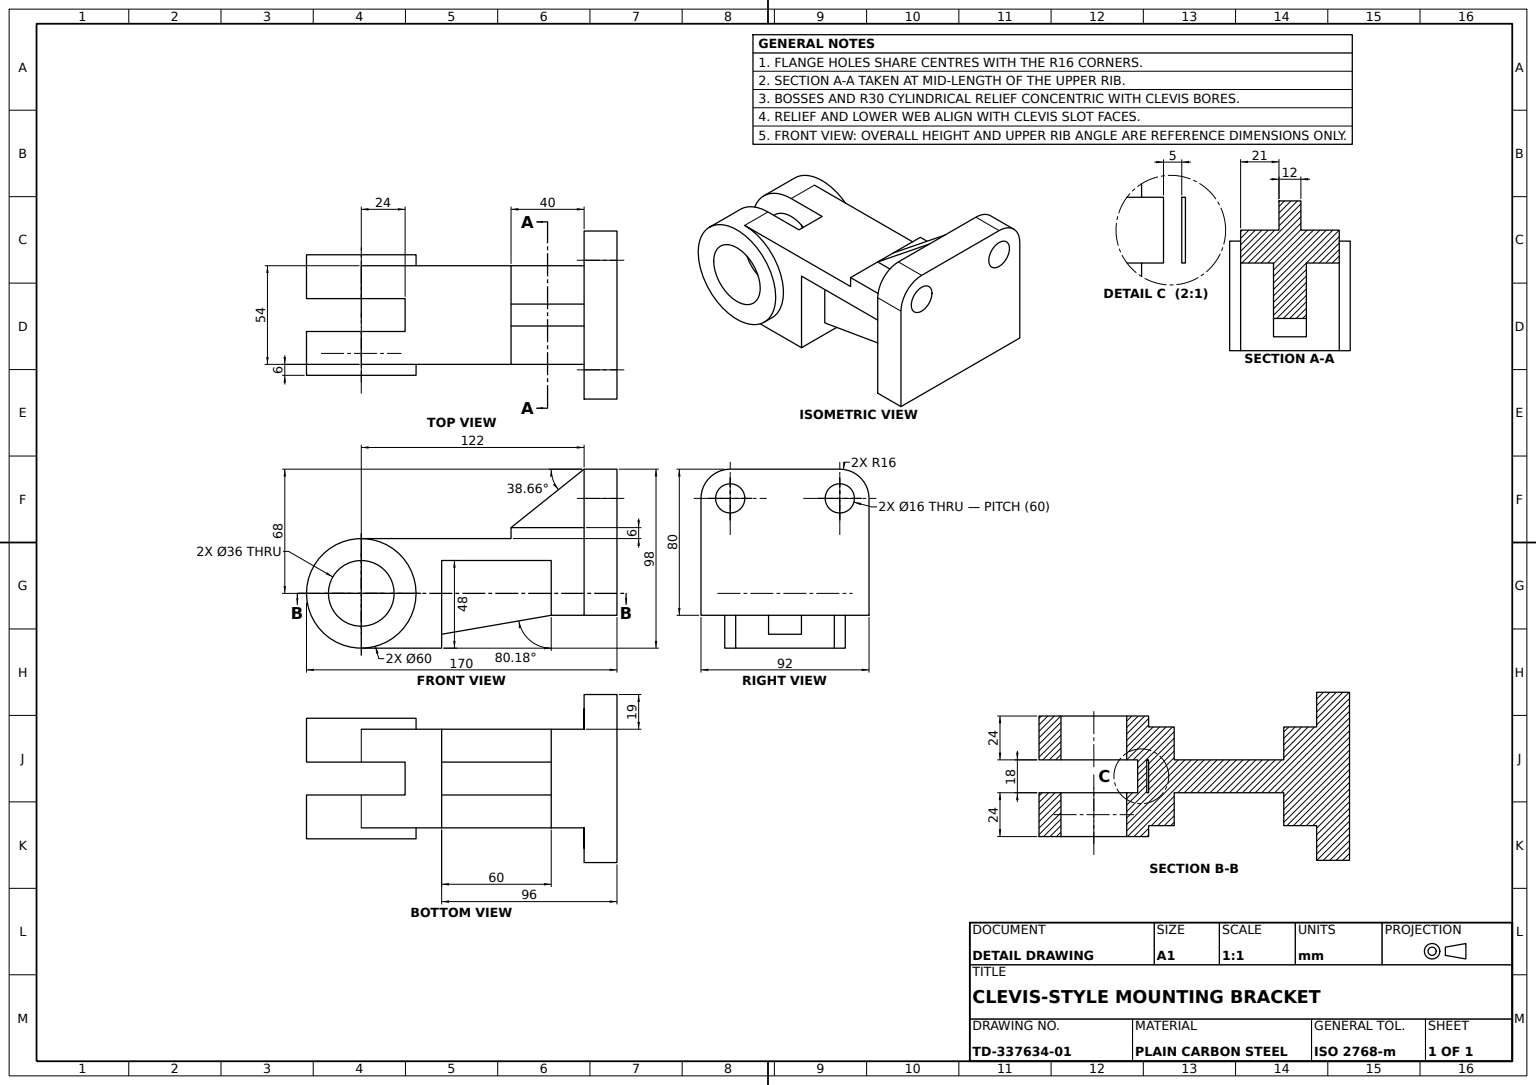
SolidWorks part; units mm, degrees
material "Plain Carbon Steel"
ref_plane "Front Plane" through (0, 0, 0) normal (0, 0, 1) x (1, 0, 0)
ref_plane "Top Plane" through (0, 0, 0) normal (0, 1, 0) x (1, 0, 0)
ref_plane "Right Plane" through (0, 0, 0) normal (1, 0, 0) x (0, 0, -1)
sketch "Hub Profile Sketch" plane through (0, 0, 0) normal (0, 0, 1) x (1, 0, 0)
  circle A0 centre (0, 0) radius 30
  dimension "D1" = 60
extrude "Hub Ø60" add sketch "Hub Profile Sketch" along normal blind 24
ref_plane "Hub Offset Plane" through (0, 0, -18) normal (0, 0, -1) x (-1, 0, 0)
sketch "Hub Extension Sketch" plane through (0, 0, -18) normal (0, 0, -1) x (-1, 0, 0)
  circle A0 centre (0, 0) radius 30
  dimension "D1" = 60
extrude "Hub Extension Ø60" add sketch "Hub Extension Sketch" along normal blind 24 separate body
sketch "Hub Bore Sketch" plane through (0, 0, 24) normal (0, 0, 1) x (1, 0, 0)
  circle A0 centre (0, 0) radius 18
  dimension "D1" = 36
extrude "Hub Bore Ø36" cut sketch "Hub Bore Sketch" against normal blind 98
ref_plane "Arm Sketch Plane" through (0, 0, 18) normal (0, 0, 1) x (1, 0, 0)
sketch "Arm Profile Sketch" plane through (0, 0, 18) normal (0, 0, 1) x (1, 0, 0)
  line L0 (0, 30) -> (122, 30)
  line L1 (122, 30) -> (122, -30)
  line L2 (122, -30) -> (0, -30)
  circle A0 centre (0, 0) radius 30 construction
  arc A1 (0, -30) -> (0, 30) centre (0, 0) ccw
  dimension "D1" = 122
  dimension "D2" = 122
  dimension "D3" = 122
extrude "Arm Body" add sketch "Arm Profile Sketch" against normal blind 54
sketch "Clevis Slot Sketch" plane through (0, 30, 0) normal (0, 1, 0) x (1, 0, 0)
  line L0 (0, 0) -> (24, 0)
  line L1 (18, 0) -> (-18, 0) construction
  line L2 (24, 0) -> (24, 18)
  line L3 (24, 18) -> (0, 18)
  line L4 (0, 18) -> (0, 0)
  dimension "D1" = 24
extrude "Clevis Slot 24mm" cut sketch "Clevis Slot Sketch" against normal blind 96
sketch "Slot Pad Sketch" plane through (24, 0, 0) normal (-1, 0, 0) x (0, 0, 1)
  line L0 (-18, -30) -> (-18, 30)
  line L1 (-18, 30) -> (0, 30)
  line L2 (0, 30) -> (0, -30)
  line L3 (0, -30) -> (-18, -30)
extrude "Slot Pad 5mm" add sketch "Slot Pad Sketch" against normal blind 5
sketch "Rib Base Pad Sketch" plane through (0, 30, 0) normal (0, 1, 0) x (1, 0, 0)
  line L0 (122, -18) -> (82, -18)
  line L1 (122, -18) -> (0, -18) construction
  line L2 (82, -18) -> (82, 36)
  line L3 (122, 36) -> (0, 36) construction
  line L4 (82, 36) -> (122, 36)
  line L5 (122, 36) -> (122, -18)
  dimension "D1" = 40
extrude "Rib Base Pad" add sketch "Rib Base Pad Sketch" along normal blind 6
ref_plane "Flange Mid Plane" through (0, 0, -9) normal (0, 0, -1) x (-1, 0, 0)
sketch "Mounting Flange Sketch" plane through (0, 0, -9) normal (0, 0, -1) x (-1, 0, 0)
  line L0 (-122, 68) -> (-140, 68)
  line L1 (-122, -30) -> (-122, 36) construction
  line L2 (-122, -12) -> (-122, 68)
  line L3 (-140, 68) -> (-140, -12)
  line L4 (-140, -12) -> (-122, -12)
  dimension "D1" = 80
  dimension "D2" = 18
  dimension "D3" = 68
extrude "Mounting Flange" add sketch "Mounting Flange Sketch" along normal mid plane 92
fillet "Flange Corner Fillet R16 A" radius 16 1 edges at (131, 68, 37)
fillet "Flange Corner Fillet R16 B" radius 16 1 edges at (131, 68, -55)
sketch "Flange Holes Sketch" plane through (122, 0, 0) normal (-1, 0, 0) x (0, 0, 1)
  circle A0 centre (21, 52) radius 8
  circle A1 centre (-39, 52) radius 8
  dimension "D1" = 16
  dimension "D2" = 16
extrude "Flange Holes 2xØ16" cut sketch "Flange Holes Sketch" against normal blind 92
sketch "Flange Rib Sketch" plane through (0, 0, -9) normal (0, 0, -1) x (-1, 0, 0)
  line L0 (-82, 36) -> (-122, 68)
rib "Flange Rib 12mm" sketch "Flange Rib Sketch" sketch "Flange Rib Sketch" thickness 12 extrusion direction parallel to sketch draft on no parameters "D1"=12
sketch "Arm Relief Sketch" plane through (0, 0, 18) normal (0, 0, 1) x (1, 0, 0)
  line L0 (122, -12) -> (104, -12)
  line L1 (122, -30) -> (44, -30)
  line L2 (0, -30) -> (122, -30) construction
  line L3 (44, -30) -> (104, -12)
  line L4 (122, -30) -> (122, -12)
  line L5 (44, -30) -> (44, 18)
  line L6 (44, 18) -> (104, 18)
  line L7 (104, 18) -> (104, -12)
  line M6 (0, -30) -> (122, -30)
  line M7 (122, -30) -> (122, -12)
  dimension "D1" = 60
  dimension "D2" = 48
extrude "Arm Relief Cut" cut sketch "Arm Relief Sketch" against normal blind 92 contours L7 L6 L5 L3 | L3 L0 M6 M7
sketch "Arm Rib Sketch" plane through (0, 0, -9) normal (0, 0, -1) x (-1, 0, 0)
  line L0 (0, -30) -> (-104, -12)
rib "Arm Rib 18mm" sketch "Arm Rib Sketch" sketch "Arm Rib Sketch" thickness 18 extrusion direction parallel to sketch draft on no parameters "D1"=18
